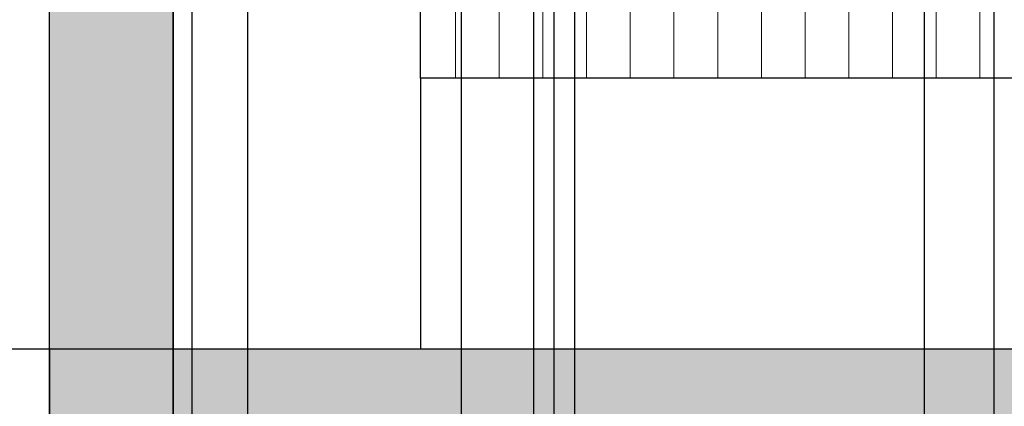
# Model space of a CAD drawing. Units: inches. Extents: x 241 to 943, y 109 to 1396.
# Tile 21 of 34: x 374 to 470, y 1065 to 1103. Entities that reach past the tile are written whole.
import ezdxf

# ---------------------------------------------------------------- set-up
doc = ezdxf.new("R2010")
doc.units = ezdxf.units.IN
doc.header["$MEASUREMENT"] = 0
for name, color, linetype, lineweight in [('A-ANNO-DIMS', 2, 'Continuous', 18), ('A-ELEV', 7, 'Continuous', 25), ('A-ELEV-SHAD', 9, 'Continuous', 13), ('A-GLAZ-PATT', 18, 'Continuous', 13), ('A-WALL-PATT', 8, 'Continuous', 13)]:
    doc.layers.add(name, color=color, linetype=linetype, lineweight=lineweight)
doc.styles.get("Standard").update_dxf_attribs({"font": 'arial.ttf'})
doc.dimstyles.get("Standard").update_dxf_attribs({"dimtxt": 1.4375, "dimasz": 0.18, "dimexe": 0.18, "dimexo": 0.0625, "dimgap": 0.09, "dimtad": 0, "dimtih": 1, "dimtoh": 1, "dimdec": 4, "dimzin": 0, "dimdsep": 46, "dimlunit": 4, "dimtxsty": 'Standard', "dimcen": 0.09, "dimadec": 0, "dimazin": 0, "dimtfac": 1, "dimtdec": 4, "dimtofl": 0, "dimtmove": 0, "dimatfit": 3, "dimfxl": 1, "dimtolj": 1, "dimtzin": 0, "dimarcsym": 0})

# ---------------------------------------------------------------- blocks, each defined once
blk = doc.blocks.new('BALCONY-RAIL')
for p, q in [((26.076, 26.374), (26.076, 52.061)), ((99.299, 26.374), (26.076, 26.374)), ((26.076, 26.374), (26.076, 0))]:
    blk.add_line(p, q)
blk = doc.blocks.new('*D5')
at = {"layer": 'A-ANNO-DIMS', "color": 0, "lineweight": -2, "transparency": 16777216}
for p, q in [((303.236, 177.803), (303.236, 1395.045)), ((377.039, 177.76), (377.039, 1395.045)), ((303.416, 1394.865), (338.185, 1394.865)), ((376.859, 1394.865), (342.09, 1394.865))]:
    blk.add_line(p, q, dxfattribs=at)
at = {"layer": 'A-ANNO-DIMS', "color": 0, "transparency": 16777216}
for points in [[(303.416, 1394.895), (303.416, 1394.835), (303.236, 1394.865)], [(376.859, 1394.895), (376.859, 1394.835), (377.039, 1394.865)]]:
    blk.add_solid(points, dxfattribs=at)
at = {"layer": 'Defpoints', "color": 0, "transparency": 16777216}
for p in [(377.039, 1394.865), (303.236, 177.741), (377.039, 177.698)]:
    blk.add_point(p, dxfattribs=at)
at = {"layer": 'A-ANNO-DIMS', "color": 0, "transparency": 16777216, "insert": (340.137, 1394.865), "char_height": 1.4375, "attachment_point": 5}
blk.add_mtext('\\A1;73.8', dxfattribs=at)
blk = doc.blocks.new('*D7')
at = {"layer": 'A-ANNO-DIMS', "color": 0, "lineweight": -2, "transparency": 16777216}
for p, q in [((508.244, 1336.115), (244.306, 1336.115)), ((244.486, 1335.935), (244.486, 753.252)), ((244.486, 168.921), (244.486, 751.604)), ((303.173, 168.741), (244.306, 168.741))]:
    blk.add_line(p, q, dxfattribs=at)
at = {"layer": 'A-ANNO-DIMS', "color": 0, "transparency": 16777216}
for points in [[(244.456, 1335.935), (244.516, 1335.935), (244.486, 1336.115)], [(244.456, 168.921), (244.516, 168.921), (244.486, 168.741)]]:
    blk.add_solid(points, dxfattribs=at)
at = {"layer": 'Defpoints', "color": 0, "transparency": 16777216}
for p in [(244.486, 1336.115), (508.306, 1336.115), (303.236, 168.741)]:
    blk.add_point(p, dxfattribs=at)
at = {"layer": 'A-ANNO-DIMS', "color": 0, "transparency": 16777216, "insert": (244.486, 752.428), "char_height": 1.4375, "attachment_point": 5}
blk.add_mtext('\\A1;1167.4', dxfattribs=at)
blk = doc.blocks.new('*D8')
at = {"layer": 'A-ANNO-DIMS', "color": 0, "lineweight": -2, "transparency": 16777216}
for p, q in [((377.039, 396.941), (377.039, 1395.045)), ((390.895, 384.241), (390.895, 1395.045)), ((377.219, 1394.865), (380.961, 1394.865)), ((390.715, 1394.865), (386.973, 1394.865))]:
    blk.add_line(p, q, dxfattribs=at)
at = {"layer": 'A-ANNO-DIMS', "color": 0, "transparency": 16777216}
for points in [[(377.219, 1394.895), (377.219, 1394.835), (377.039, 1394.865)], [(390.715, 1394.895), (390.715, 1394.835), (390.895, 1394.865)]]:
    blk.add_solid(points, dxfattribs=at)
at = {"layer": 'Defpoints', "color": 0, "transparency": 16777216}
for p in [(390.895, 1394.865), (377.039, 396.878), (390.895, 384.178)]:
    blk.add_point(p, dxfattribs=at)
at = {"layer": 'A-ANNO-DIMS', "color": 0, "transparency": 16777216, "insert": (383.967, 1394.865), "char_height": 1.4375, "attachment_point": 5}
blk.add_mtext('\\A1;13.856', dxfattribs=at)
blk = doc.blocks.new('*D9')
at = {"layer": 'A-ANNO-DIMS', "color": 0, "lineweight": -2, "transparency": 16777216}
for p, q in [((390.895, 384.241), (390.895, 1395.045)), ((462.107, 384.241), (462.107, 1395.045)), ((391.075, 1394.865), (424.13, 1394.865)), ((461.927, 1394.865), (428.872, 1394.865))]:
    blk.add_line(p, q, dxfattribs=at)
at = {"layer": 'A-ANNO-DIMS', "color": 0, "transparency": 16777216}
for points in [[(391.075, 1394.895), (391.075, 1394.835), (390.895, 1394.865)], [(461.927, 1394.895), (461.927, 1394.835), (462.107, 1394.865)]]:
    blk.add_solid(points, dxfattribs=at)
at = {"layer": 'Defpoints', "color": 0, "transparency": 16777216}
for p in [(462.107, 1394.865), (390.895, 384.178), (462.107, 384.178)]:
    blk.add_point(p, dxfattribs=at)
at = {"layer": 'A-ANNO-DIMS', "color": 0, "transparency": 16777216, "insert": (426.501, 1394.865), "char_height": 1.4375, "attachment_point": 5}
blk.add_mtext('\\A1;71.21', dxfattribs=at)
blk = doc.blocks.new('*D10')
at = {"layer": 'A-ANNO-DIMS', "color": 0, "lineweight": -2, "transparency": 16777216}
for p, q in [((462.107, 384.241), (462.107, 1395.045)), ((479.596, 384.241), (479.596, 1395.045)), ((462.287, 1394.865), (468.402, 1394.865)), ((479.416, 1394.865), (473.301, 1394.865))]:
    blk.add_line(p, q, dxfattribs=at)
at = {"layer": 'A-ANNO-DIMS', "color": 0, "transparency": 16777216}
for points in [[(462.287, 1394.895), (462.287, 1394.835), (462.107, 1394.865)], [(479.416, 1394.895), (479.416, 1394.835), (479.596, 1394.865)]]:
    blk.add_solid(points, dxfattribs=at)
at = {"layer": 'Defpoints', "color": 0, "transparency": 16777216}
for p in [(479.596, 1394.865), (462.107, 384.178), (479.596, 384.178)]:
    blk.add_point(p, dxfattribs=at)
at = {"layer": 'A-ANNO-DIMS', "color": 0, "transparency": 16777216, "insert": (470.852, 1394.865), "char_height": 1.4375, "attachment_point": 5}
blk.add_mtext('\\A1;17.49', dxfattribs=at)
blk = doc.blocks.new('*D25')
at = {"layer": 'A-ANNO-DIMS', "color": 0, "lineweight": -2, "transparency": 16777216}
for p, q in [((376.977, 1070.854), (244.306, 1070.854)), ((244.486, 1070.674), (244.486, 1041.02)), ((244.486, 1009.718), (244.486, 1039.372)), ((376.977, 1009.538), (244.306, 1009.538))]:
    blk.add_line(p, q, dxfattribs=at)
at = {"layer": 'A-ANNO-DIMS', "color": 0, "transparency": 16777216}
for points in [[(244.456, 1070.674), (244.516, 1070.674), (244.486, 1070.854)], [(244.456, 1009.718), (244.516, 1009.718), (244.486, 1009.538)]]:
    blk.add_solid(points, dxfattribs=at)
at = {"layer": 'Defpoints', "color": 0, "transparency": 16777216}
for p in [(244.486, 1070.854), (377.039, 1070.854), (377.039, 1009.538)]:
    blk.add_point(p, dxfattribs=at)
at = {"layer": 'A-ANNO-DIMS', "color": 0, "transparency": 16777216, "insert": (244.486, 1040.196), "char_height": 1.4375, "attachment_point": 5}
blk.add_mtext('\\A1;61.32', dxfattribs=at)
blk = doc.blocks.new('*D26')
at = {"layer": 'A-ANNO-DIMS', "color": 0, "lineweight": -2, "transparency": 16777216}
for p, q in [((376.977, 1177.538), (244.306, 1177.538)), ((244.486, 1177.358), (244.486, 1125.02)), ((244.486, 1071.034), (244.486, 1123.372)), ((376.977, 1070.854), (244.306, 1070.854))]:
    blk.add_line(p, q, dxfattribs=at)
at = {"layer": 'A-ANNO-DIMS', "color": 0, "transparency": 16777216}
for points in [[(244.456, 1177.358), (244.516, 1177.358), (244.486, 1177.538)], [(244.456, 1071.034), (244.516, 1071.034), (244.486, 1070.854)]]:
    blk.add_solid(points, dxfattribs=at)
at = {"layer": 'Defpoints', "color": 0, "transparency": 16777216}
for p in [(244.486, 1177.538), (377.039, 1177.538), (377.039, 1070.854)]:
    blk.add_point(p, dxfattribs=at)
at = {"layer": 'A-ANNO-DIMS', "color": 0, "transparency": 16777216, "insert": (244.486, 1124.196), "char_height": 1.4375, "attachment_point": 5}
blk.add_mtext('\\A1;106.68', dxfattribs=at)
blk = doc.blocks.new('*D39')
at = {"layer": 'A-ANNO-DIMS', "color": 0, "lineweight": -2, "transparency": 16777216}
for p, q in [((388.98, 1109.492), (244.306, 1109.492)), ((244.486, 1109.312), (244.486, 1090.997)), ((244.486, 1071.034), (244.486, 1089.348)), ((388.98, 1070.854), (244.306, 1070.854))]:
    blk.add_line(p, q, dxfattribs=at)
at = {"layer": 'A-ANNO-DIMS', "color": 0, "transparency": 16777216}
for points in [[(244.456, 1109.312), (244.516, 1109.312), (244.486, 1109.492)], [(244.456, 1071.034), (244.516, 1071.034), (244.486, 1070.854)]]:
    blk.add_solid(points, dxfattribs=at)
at = {"layer": 'Defpoints', "color": 0, "transparency": 16777216}
for p in [(244.486, 1109.492), (389.043, 1109.492), (389.043, 1070.854)]:
    blk.add_point(p, dxfattribs=at)
at = {"layer": 'A-ANNO-DIMS', "color": 0, "transparency": 16777216, "insert": (244.486, 1090.173), "char_height": 1.4375, "attachment_point": 5}
blk.add_mtext('\\A1;38.64', dxfattribs=at)
blk = doc.blocks.new('*D61')
at = {"layer": 'A-ANNO-DIMS', "color": 0, "lineweight": -2, "transparency": 16777216}
for p, q in [((377.039, 400.892), (377.039, 1395.045)), ((424.109, 568.892), (424.109, 1395.045)), ((377.219, 1394.865), (398.03, 1394.865)), ((423.929, 1394.865), (403.118, 1394.865))]:
    blk.add_line(p, q, dxfattribs=at)
at = {"layer": 'A-ANNO-DIMS', "color": 0, "transparency": 16777216}
for points in [[(377.219, 1394.895), (377.219, 1394.835), (377.039, 1394.865)], [(423.929, 1394.895), (423.929, 1394.835), (424.109, 1394.865)]]:
    blk.add_solid(points, dxfattribs=at)
at = {"layer": 'Defpoints', "color": 0, "transparency": 16777216}
for p in [(424.109, 1394.865), (424.109, 568.829), (377.039, 400.829)]:
    blk.add_point(p, dxfattribs=at)
at = {"layer": 'A-ANNO-DIMS', "color": 0, "transparency": 16777216, "insert": (400.574, 1394.865), "char_height": 1.4375, "attachment_point": 5}
blk.add_mtext('\\A1;47.07', dxfattribs=at)
blk = doc.blocks.new('*D62')
at = {"layer": 'A-ANNO-DIMS', "color": 0, "lineweight": -2, "transparency": 16777216}
for p, q in [((424.109, 568.892), (424.109, 1395.045)), ((565.202, 568.892), (565.202, 1395.045)), ((424.289, 1394.865), (492.346, 1394.865)), ((565.022, 1394.865), (496.964, 1394.865))]:
    blk.add_line(p, q, dxfattribs=at)
at = {"layer": 'A-ANNO-DIMS', "color": 0, "transparency": 16777216}
for points in [[(424.289, 1394.895), (424.289, 1394.835), (424.109, 1394.865)], [(565.022, 1394.895), (565.022, 1394.835), (565.202, 1394.865)]]:
    blk.add_solid(points, dxfattribs=at)
at = {"layer": 'Defpoints', "color": 0, "transparency": 16777216}
for p in [(565.202, 1394.865), (424.109, 568.829), (565.202, 568.829)]:
    blk.add_point(p, dxfattribs=at)
at = {"layer": 'A-ANNO-DIMS', "color": 0, "transparency": 16777216, "insert": (494.655, 1394.865), "char_height": 1.4375, "attachment_point": 5}
blk.add_mtext('\\A1;141.1', dxfattribs=at)
blk = doc.blocks.new('*D65')
at = {"layer": 'A-ANNO-DIMS', "color": 0, "lineweight": -2, "transparency": 16777216}
for p, q in [((424.109, 700.854), (424.109, 1395.045)), ((592.954, 700.854), (592.954, 1395.045)), ((424.289, 1394.865), (505.52, 1394.865)), ((592.774, 1394.865), (511.543, 1394.865))]:
    blk.add_line(p, q, dxfattribs=at)
at = {"layer": 'A-ANNO-DIMS', "color": 0, "transparency": 16777216}
for points in [[(424.289, 1394.895), (424.289, 1394.835), (424.109, 1394.865)], [(592.774, 1394.895), (592.774, 1394.835), (592.954, 1394.865)]]:
    blk.add_solid(points, dxfattribs=at)
at = {"layer": 'Defpoints', "color": 0, "transparency": 16777216}
for p in [(592.954, 1394.865), (424.109, 700.791), (592.954, 700.791)]:
    blk.add_point(p, dxfattribs=at)
at = {"layer": 'A-ANNO-DIMS', "color": 0, "transparency": 16777216, "insert": (508.531, 1394.865), "char_height": 1.4375, "attachment_point": 5}
blk.add_mtext('\\A1;168.85', dxfattribs=at)
blk = doc.blocks.new('*D67')
at = {"layer": 'A-ANNO-DIMS', "color": 0, "lineweight": -2, "transparency": 16777216}
for p, q in [((389.043, 773.554), (389.043, 1395.045)), ((607.816, 773.554), (607.816, 1395.045)), ((389.223, 1394.865), (495.343, 1394.865)), ((607.636, 1394.865), (501.516, 1394.865))]:
    blk.add_line(p, q, dxfattribs=at)
at = {"layer": 'A-ANNO-DIMS', "color": 0, "transparency": 16777216}
for points in [[(389.223, 1394.895), (389.223, 1394.835), (389.043, 1394.865)], [(607.636, 1394.895), (607.636, 1394.835), (607.816, 1394.865)]]:
    blk.add_solid(points, dxfattribs=at)
at = {"layer": 'Defpoints', "color": 0, "transparency": 16777216}
for p in [(607.816, 1394.865), (389.043, 773.492), (607.816, 773.492)]:
    blk.add_point(p, dxfattribs=at)
at = {"layer": 'A-ANNO-DIMS', "color": 0, "transparency": 16777216, "insert": (498.43, 1394.865), "char_height": 1.4375, "attachment_point": 5}
blk.add_mtext('\\A1;218.77', dxfattribs=at)
blk = doc.blocks.new('*D69')
at = {"layer": 'A-ANNO-DIMS', "color": 0, "lineweight": -2, "transparency": 16777216}
for p, q in [((389.043, 941.554), (389.043, 1395.045)), ((568.135, 941.554), (568.135, 1395.045)), ((389.223, 1394.865), (476.28, 1394.865)), ((567.955, 1394.865), (480.898, 1394.865))]:
    blk.add_line(p, q, dxfattribs=at)
at = {"layer": 'A-ANNO-DIMS', "color": 0, "transparency": 16777216}
for points in [[(389.223, 1394.895), (389.223, 1394.835), (389.043, 1394.865)], [(567.955, 1394.895), (567.955, 1394.835), (568.135, 1394.865)]]:
    blk.add_solid(points, dxfattribs=at)
at = {"layer": 'Defpoints', "color": 0, "transparency": 16777216}
for p in [(568.135, 1394.865), (389.043, 941.492), (568.135, 941.492)]:
    blk.add_point(p, dxfattribs=at)
at = {"layer": 'A-ANNO-DIMS', "color": 0, "transparency": 16777216, "insert": (478.589, 1394.865), "char_height": 1.4375, "attachment_point": 5}
blk.add_mtext('\\A1;179.1', dxfattribs=at)
blk = doc.blocks.new('*D89')
at = {"layer": 'A-ANNO-DIMS', "color": 0, "lineweight": -2, "transparency": 16777216}
for p, q in [((377.039, 841.601), (377.039, 1395.045)), ((617.759, 841.601), (617.759, 1395.045)), ((377.219, 1394.865), (494.321, 1394.865)), ((617.579, 1394.865), (500.478, 1394.865))]:
    blk.add_line(p, q, dxfattribs=at)
at = {"layer": 'A-ANNO-DIMS', "color": 0, "transparency": 16777216}
for points in [[(377.219, 1394.895), (377.219, 1394.835), (377.039, 1394.865)], [(617.579, 1394.895), (617.579, 1394.835), (617.759, 1394.865)]]:
    blk.add_solid(points, dxfattribs=at)
at = {"layer": 'Defpoints', "color": 0, "transparency": 16777216}
for p in [(617.759, 1394.865), (377.039, 841.538), (617.759, 841.538)]:
    blk.add_point(p, dxfattribs=at)
at = {"layer": 'A-ANNO-DIMS', "color": 0, "transparency": 16777216, "insert": (497.399, 1394.865), "char_height": 1.4375, "attachment_point": 5}
blk.add_mtext('\\A1;240.72', dxfattribs=at)
blk = doc.blocks.new('*D91')
at = {"layer": 'A-ANNO-DIMS', "color": 0, "lineweight": -2, "transparency": 16777216}
for p, q in [((377.039, 1070.791), (377.039, 109.811)), ((389.043, 1070.791), (389.043, 109.811)), ((377.219, 109.991), (380.038, 109.991)), ((388.863, 109.991), (386.044, 109.991))]:
    blk.add_line(p, q, dxfattribs=at)
at = {"layer": 'A-ANNO-DIMS', "color": 0, "transparency": 16777216}
for points in [[(377.219, 110.021), (377.219, 109.961), (377.039, 109.991)], [(388.863, 110.021), (388.863, 109.961), (389.043, 109.991)]]:
    blk.add_solid(points, dxfattribs=at)
at = {"layer": 'Defpoints', "color": 0, "transparency": 16777216}
for p in [(377.039, 1070.854), (389.043, 1070.854), (389.043, 109.991)]:
    blk.add_point(p, dxfattribs=at)
at = {"layer": 'A-ANNO-DIMS', "color": 0, "transparency": 16777216, "insert": (383.041, 109.991), "char_height": 1.4375, "attachment_point": 5}
blk.add_mtext('\\A1;12.004', dxfattribs=at)
blk = doc.blocks.new('*D92')
at = {"layer": 'A-ANNO-DIMS', "color": 0, "lineweight": -2, "transparency": 16777216}
for p, q in [((508.244, 1336.115), (244.306, 1336.115)), ((244.486, 1335.935), (244.486, 1204.309)), ((244.486, 1071.034), (244.486, 1202.661)), ((508.244, 1070.854), (244.306, 1070.854))]:
    blk.add_line(p, q, dxfattribs=at)
at = {"layer": 'A-ANNO-DIMS', "color": 0, "transparency": 16777216}
for points in [[(244.456, 1335.935), (244.516, 1335.935), (244.486, 1336.115)], [(244.456, 1071.034), (244.516, 1071.034), (244.486, 1070.854)]]:
    blk.add_solid(points, dxfattribs=at)
at = {"layer": 'Defpoints', "color": 0, "transparency": 16777216}
for p in [(244.486, 1336.115), (508.306, 1336.115), (508.306, 1070.854)]:
    blk.add_point(p, dxfattribs=at)
at = {"layer": 'A-ANNO-DIMS', "color": 0, "transparency": 16777216, "insert": (244.486, 1203.485), "char_height": 1.4375, "attachment_point": 5}
blk.add_mtext('\\A1;265.26', dxfattribs=at)
blk = doc.blocks.new('*D99')
at = {"layer": 'A-ANNO-DIMS', "color": 0, "lineweight": -2, "transparency": 16777216}
for p, q in [((417.091, 181.712), (417.091, 1395.045)), ((667.393, 214.581), (667.393, 1395.045)), ((417.271, 1394.865), (539.159, 1394.865)), ((667.213, 1394.865), (545.326, 1394.865))]:
    blk.add_line(p, q, dxfattribs=at)
at = {"layer": 'A-ANNO-DIMS', "color": 0, "transparency": 16777216}
for points in [[(417.271, 1394.895), (417.271, 1394.835), (417.091, 1394.865)], [(667.213, 1394.895), (667.213, 1394.835), (667.393, 1394.865)]]:
    blk.add_solid(points, dxfattribs=at)
at = {"layer": 'Defpoints', "color": 0, "transparency": 16777216}
for p in [(667.393, 1394.865), (667.393, 214.519), (417.091, 181.649)]:
    blk.add_point(p, dxfattribs=at)
at = {"layer": 'A-ANNO-DIMS', "color": 0, "transparency": 16777216, "insert": (542.242, 1394.865), "char_height": 1.4375, "attachment_point": 5}
blk.add_mtext('\\A1;250.30', dxfattribs=at)
blk = doc.blocks.new('*D101')
at = {"layer": 'A-ANNO-DIMS', "color": 0, "lineweight": -2, "transparency": 16777216}
for p, q in [((396.312, 1009.601), (396.312, 1395.045)), ((426.117, 1007.601), (426.117, 1395.045)), ((396.492, 1394.865), (408.123, 1394.865)), ((425.937, 1394.865), (414.306, 1394.865))]:
    blk.add_line(p, q, dxfattribs=at)
at = {"layer": 'A-ANNO-DIMS', "color": 0, "transparency": 16777216}
for points in [[(396.492, 1394.895), (396.492, 1394.835), (396.312, 1394.865)], [(425.937, 1394.895), (425.937, 1394.835), (426.117, 1394.865)]]:
    blk.add_solid(points, dxfattribs=at)
at = {"layer": 'Defpoints', "color": 0, "transparency": 16777216}
for p in [(426.117, 1394.865), (396.312, 1009.538), (426.117, 1007.538)]:
    blk.add_point(p, dxfattribs=at)
at = {"layer": 'A-ANNO-DIMS', "color": 0, "transparency": 16777216, "insert": (411.215, 1394.865), "char_height": 1.4375, "attachment_point": 5}
blk.add_mtext('\\A1;29.805', dxfattribs=at)
blk = doc.blocks.new('*D102')
at = {"layer": 'A-ANNO-DIMS', "color": 0, "lineweight": -2, "transparency": 16777216}
for p, q in [((428.117, 1007.601), (428.117, 1395.045)), ((468.869, 1007.601), (468.869, 1395.045)), ((428.297, 1394.865), (445.944, 1394.865)), ((468.689, 1394.865), (451.043, 1394.865))]:
    blk.add_line(p, q, dxfattribs=at)
at = {"layer": 'A-ANNO-DIMS', "color": 0, "transparency": 16777216}
for points in [[(428.297, 1394.895), (428.297, 1394.835), (428.117, 1394.865)], [(468.689, 1394.895), (468.689, 1394.835), (468.869, 1394.865)]]:
    blk.add_solid(points, dxfattribs=at)
at = {"layer": 'Defpoints', "color": 0, "transparency": 16777216}
for p in [(468.869, 1394.865), (428.117, 1007.538), (468.869, 1007.538)]:
    blk.add_point(p, dxfattribs=at)
at = {"layer": 'A-ANNO-DIMS', "color": 0, "transparency": 16777216, "insert": (448.493, 1394.865), "char_height": 1.4375, "attachment_point": 5}
blk.add_mtext('\\A1;40.75', dxfattribs=at)

msp = doc.modelspace()

# ---------------------------------------------------------------- hatches: boundary and pattern name
at = {"layer": 'A-ELEV-SHAD'}
h = msp.add_hatch(color=256, dxfattribs=at)
h.dxf.hatch_style = 1
h.paths.add_polyline_path([(508.3064, 1070.8538), (377.0391, 1070.8538), (377.0391, 1009.5382), (508.3064, 1009.5382)])
h.paths.add_polyline_path([(508.3064, 1238.8538), (377.0391, 1238.8538), (377.0391, 1177.5382), (508.3064, 1177.5382)])
h.paths.add_polyline_path([(581.3632, 902.8538), (568.1348, 902.8538), (553.5166, 902.8538), (377.0391, 902.8538), (377.0391, 841.5382), (553.5166, 841.5382), (564.8076, 841.5382), (581.3632, 841.5382)])
h.paths.add_polyline_path([(820.8374, 1275.9142), (747.7579, 1275.9142), (747.7579, 1238.8538), (820.8374, 1238.8538)])
h.paths.add_polyline_path([(820.8374, 1238.8538), (747.7579, 1238.8538), (747.9341, 1223.0633), (820.8374, 1223.0633)])
h.paths.add_polyline_path([(396.3125, 841.5382), (377.0391, 841.5382), (377.0391, 734.8538), (389.0429, 734.8538), (389.0429, 735.188), (389.0429, 773.4916), (396.3125, 773.4916), (396.3125, 780.5808), (390.5597, 780.5808), (388.0428, 780.5808, -1), (388.0428, 782.5808), (390.5597, 782.5808), (396.3125, 782.5808)])
h = msp.add_hatch(color=256, dxfattribs=at)
h.dxf.hatch_style = 1
h.paths.add_polyline_path([(396.3125, 1177.5382), (377.0391, 1177.5382), (377.0391, 1070.8538), (389.0429, 1070.8538), (389.0429, 1109.4916), (396.3125, 1109.4916), (396.3125, 1116.5808), (390.5597, 1116.5808), (388.0428, 1116.5808, -1), (388.0428, 1118.5808), (390.5597, 1118.5808), (396.3125, 1118.5808)])
at = {"layer": 'A-GLAZ-PATT'}
h = msp.add_hatch(dxfattribs=at)
h.set_pattern_fill('ANSI31', color=256, scale=34, angle=45)
h.paths.add_polyline_path([(486.3418, 786.9154), (413.1187, 786.9154), (413.1187, 761.2284), (486.3418, 761.2284)])
h.paths.add_polyline_path([(486.3418, 954.9154), (413.1187, 954.9154), (413.1187, 929.2284), (486.3418, 929.2284)])
h.paths.add_polyline_path([(462.1074, 289.6933), (390.895, 289.6933), (390.895, 277.4626), (390.895, 274.3507), (462.1074, 274.3507), (462.1074, 277.4626)])
h.paths.add_polyline_path([(500.3323, 289.6933), (479.596, 289.6933), (479.596, 274.3507), (500.3323, 274.3507)])
h.paths.add_polyline_path([(450.9259, 566.8295), (426.1086, 566.8295), (426.1086, 498.4395), (446.4348, 498.4395), (446.4348, 519.3754), (450.9259, 519.3754), (450.9259, 525.3816), (445.5808, 525.3816, -1), (445.5808, 527.3816), (450.9259, 527.3816)])
h.paths.add_polyline_path([(563.2023, 508.9074), (534.1778, 508.9074), (508.1906, 508.9074), (508.1906, 498.4395), (563.2023, 498.4395)])
h.paths.add_polyline_path([(747.6328, 700.7912), (712.0171, 700.7912), (712.0171, 628.4013), (747.6328, 628.4013)])
h.paths.add_polyline_path([(446.4348, 643.7483), (426.1086, 643.7483), (426.1086, 630.4013), (446.4348, 630.4013)])
h.paths.add_polyline_path([(564.8076, 841.5382), (553.5166, 841.5382), (508.3064, 841.5382), (508.3064, 782.5808), (564.8076, 782.5808)])
h.paths.add_polyline_path([(564.8076, 780.5808), (508.3064, 780.5808), (508.3064, 773.4916), (564.8076, 773.4916)])
h.paths.add_polyline_path([(792.691, 762.5799), (759.6248, 762.5799), (759.6248, 736.9235), (759.6248, 734.8538), (792.691, 734.8538)])
h.paths.add_polyline_path([(564.8076, 1009.5382), (553.5166, 1009.5382), (508.3064, 1009.5382), (508.3064, 950.5808), (562.3033, 950.5808, -1), (562.3033, 948.5808), (508.3064, 948.5808), (508.3064, 941.4916), (564.8076, 941.4916)])
h.paths.add_polyline_path([(486.3418, 1122.9154), (413.1187, 1122.9154), (413.1187, 1097.2284), (486.3418, 1097.2284)])
at = {"layer": 'A-WALL-PATT'}
h = msp.add_hatch(dxfattribs=at)
h.set_pattern_fill('GRATE', color=256, scale=150)
h.paths.add_polyline_path([(747.7579, 1238.8538), (747.7579, 1275.9142), (747.7579, 1336.1154), (508.3064, 1336.1154), (508.3064, 1275.9142), (508.3064, 1238.8538), (508.3064, 1177.5382), (508.3064, 1109.4916), (508.3064, 1070.8538), (553.5166, 1070.8538), (749.6328, 1070.8538)])
h.paths.add_polyline_path([(533.952, 1108.1686), (533.952, 1177.7336), (533.952, 1303.0286), (724.819, 1303.0286), (724.819, 1108.1686)], flags=16)
h.paths.add_polyline_path([(535.952, 1110.1686), (535.952, 1175.7336), (722.819, 1175.7336), (722.819, 1110.1686)], flags=0)
h.paths.add_polyline_path([(643.4534, 1134.0739), (622.521, 1134.0739), (622.521, 1136.0739), (643.4534, 1136.0739)], flags=0)
h.paths.add_polyline_path([(617.7594, 568.8295), (617.7594, 734.8538), (377.0391, 734.8538), (377.0391, 566.8538), (377.0391, 400.8295), (417.0913, 400.8295), (618.9643, 400.8295)])
h.paths.add_polyline_path([(424.1086, 496.4395), (424.1086, 568.8295), (565.2023, 568.8295), (565.2023, 496.4395)], flags=16)
h.paths.add_polyline_path([(426.1086, 498.4395), (426.1086, 566.8295), (563.2023, 566.8295), (563.2023, 508.9074), (563.2023, 498.4395)], flags=0)
h.paths.add_polyline_path([(508.0803, 508.9074), (508.0803, 519.3754), (450.9259, 519.3754), (450.9259, 525.3816), (445.5808, 525.3816, -1), (445.5808, 527.3816), (450.9259, 527.3816), (450.9259, 566.8295), (508.0803, 566.8295), (537.4269, 566.8295), (537.4269, 508.9074)], flags=0)
h.paths.add_polyline_path([(506.0803, 521.3754), (452.9259, 521.3754), (452.9259, 564.8295), (506.0803, 564.8295)], flags=0)
h.paths.add_polyline_path([(424.1086, 628.4013), (424.1086, 700.7912), (592.9542, 700.7912), (592.9542, 628.4013)], flags=16)
h.paths.add_polyline_path([(426.1086, 630.4013), (426.1086, 698.7912), (590.8792, 698.7912), (590.8792, 630.4013)], flags=0)
h.paths.add_polyline_path([(508.1906, 651.3371), (508.0803, 651.3371), (450.9259, 651.3371), (428.0291, 651.3371), (428.0291, 698.7912), (451.9767, 698.7912), (508.0803, 698.7912), (537.4269, 698.7912), (563.2023, 698.7912), (563.2023, 659.3434), (563.9297, 659.3434), (563.9297, 651.3371)], flags=0)
h.paths.add_polyline_path([(506.0803, 653.3371), (452.9259, 653.3371), (452.9259, 657.3434), (445.5808, 657.3434, -1), (445.5808, 659.3434), (452.9259, 659.3434), (452.9259, 696.7912), (506.0803, 696.7912)], flags=0)

# ---------------------------------------------------------------- linework, layer by layer
at = {"layer": 'A-ELEV'}
for p, q in [((377.0391, 1070.8538), (377.0391, 1238.8538)), ((389.0429, 1109.4916), (389.0429, 1070.8538)), ((377.0391, 902.8538), (377.0391, 1070.8538)), ((553.5166, 1070.8538), (377.0391, 1070.8538))]:
    msp.add_line(p, q, dxfattribs=at)

# ---------------------------------------------------------------- block references
msp.add_blockref('BALCONY-RAIL', (387.043, 1070.854), dxfattribs=at)

# ---------------------------------------------------------------- dimensions: what is measured, and where the dimension line sits
at = {"layer": 'A-ANNO-DIMS'}
for base, p1, p2, override, picture, middle in [((377.0391, 1394.8654), (303.2358, 177.7407), (377.0391, 177.6977), {"dimdec": 1, "dimlfac": 1, "dimrnd": 0, "dimzin": 0, "dimdsep": 46, "dimlunit": 2}, '*D5', (340.1375, 1394.8654)), ((390.895, 1394.8654), (377.0391, 396.8782), (390.895, 384.1784), {"dimdec": 3, "dimlfac": 1, "dimrnd": 0, "dimzin": 0, "dimdsep": 46, "dimlunit": 2}, '*D8', (383.9671, 1394.8654)), ((424.1086, 1394.8654), (377.0391, 400.8295), (424.1086, 568.8295), {"dimdec": 2, "dimlfac": 1, "dimrnd": 0, "dimzin": 0, "dimdsep": 46, "dimlunit": 2}, '*D61', (400.5739, 1394.8654)), ((617.7594, 1394.8654), (377.0391, 841.5382), (617.7594, 841.5382), {"dimdec": 2, "dimlfac": 1, "dimrnd": 0, "dimzin": 0, "dimdsep": 46, "dimlunit": 2}, '*D89', (497.3993, 1394.8654)), ((607.8162, 1394.8654), (389.0429, 773.4916), (607.8162, 773.4916), {"dimdec": 2, "dimlfac": 1, "dimrnd": 0, "dimzin": 0, "dimdsep": 46, "dimlunit": 2}, '*D67', (498.4295, 1394.8654)), ((568.1348, 1394.8654), (389.0429, 941.4916), (568.1348, 941.4916), {"dimdec": 1, "dimlfac": 1, "dimrnd": 0, "dimzin": 0, "dimdsep": 46, "dimlunit": 2}, '*D69', (478.5888, 1394.8654)), ((462.1074, 1394.8654), (390.895, 384.1784), (462.1074, 384.1784), {"dimdec": 2, "dimlfac": 1, "dimrnd": 0, "dimzin": 0, "dimdsep": 46, "dimlunit": 2}, '*D9', (426.5012, 1394.8654)), ((426.1173, 1394.8654), (396.3125, 1009.5382), (426.1173, 1007.5382), {"dimdec": 3, "dimlfac": 1, "dimrnd": 0, "dimzin": 0, "dimdsep": 46, "dimlunit": 2}, '*D101', (411.2149, 1394.8654)), ((667.3935, 1394.8654), (417.0913, 181.649), (667.3935, 214.5189), {"dimdec": 2, "dimlfac": 1, "dimrnd": 0, "dimzin": 0, "dimdsep": 46, "dimlunit": 2}, '*D99', (542.2424, 1394.8654)), ((565.2023, 1394.8654), (424.1086, 568.8295), (565.2023, 568.8295), {"dimdec": 1, "dimlfac": 1, "dimrnd": 0, "dimzin": 0, "dimdsep": 46, "dimlunit": 2}, '*D62', (494.6554, 1394.8654)), ((592.9542, 1394.8654), (424.1086, 700.7912), (592.9542, 700.7912), {"dimdec": 2, "dimlfac": 1, "dimrnd": 0, "dimzin": 0, "dimdsep": 46, "dimlunit": 2}, '*D65', (508.5314, 1394.8654)), ((468.8692, 1394.8654), (428.1173, 1007.5382), (468.8692, 1007.5382), {"dimdec": 2, "dimlfac": 1, "dimrnd": 0, "dimzin": 0, "dimdsep": 46, "dimlunit": 2}, '*D102', (448.4933, 1394.8654)), ((479.596, 1394.8654), (462.1074, 384.1784), (479.596, 384.1784), {"dimdec": 2, "dimlfac": 1, "dimrnd": 0, "dimzin": 0, "dimdsep": 46, "dimlunit": 2}, '*D10', (470.8517, 1394.8654)), ((389.0429, 109.9907), (377.0391, 1070.8538), (389.0429, 1070.8538), {"dimdec": 3, "dimlfac": 1, "dimrnd": 0, "dimzin": 0, "dimdsep": 46, "dimlunit": 2}, '*D91', (383.041, 109.9907))]:
    dim = msp.add_linear_dim(base=base, p1=p1, p2=p2, dimstyle='Standard', override=override, dxfattribs=at)
    dim.commit()
    dim.dimension.update_dxf_attribs({"geometry": picture, "text_midpoint": middle})
for base, p1, p2, override, picture, middle in [((244.4858, 1336.1154), (303.2358, 168.7407), (508.3064, 1336.1154), {"dimdec": 1, "dimlfac": 1, "dimrnd": 0, "dimzin": 0, "dimdsep": 46, "dimlunit": 2}, '*D7', (244.4858, 752.4281)), ((244.4858, 1336.1154), (508.3064, 1070.8538), (508.3064, 1336.1154), {"dimdec": 2, "dimlfac": 1, "dimrnd": 0, "dimzin": 0, "dimdsep": 46, "dimlunit": 2}, '*D92', (244.4858, 1203.4846)), ((244.4858, 1177.5382), (377.0391, 1070.8538), (377.0391, 1177.5382), {"dimdec": 2, "dimlfac": 1, "dimrnd": 0, "dimzin": 0, "dimdsep": 46, "dimlunit": 2}, '*D26', (244.4858, 1124.196)), ((244.4858, 1109.4916), (389.0429, 1070.8538), (389.0429, 1109.4916), {"dimdec": 2, "dimlfac": 1, "dimrnd": 0, "dimzin": 0, "dimdsep": 46, "dimlunit": 2}, '*D39', (244.4858, 1090.1727)), ((244.4858, 1070.8538), (377.0391, 1009.5382), (377.0391, 1070.8538), {"dimdec": 2, "dimlfac": 1, "dimrnd": 0, "dimzin": 0, "dimdsep": 46, "dimlunit": 2}, '*D25', (244.4858, 1040.196))]:
    dim = msp.add_linear_dim(base=base, p1=p1, p2=p2, angle=90, dimstyle='Standard', override=override, dxfattribs=at)
    dim.commit()
    dim.dimension.update_dxf_attribs({"geometry": picture, "text_midpoint": middle})

doc.saveas('drawing.dxf')
